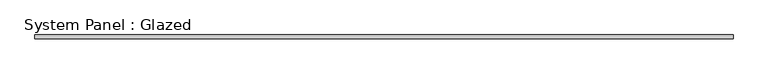
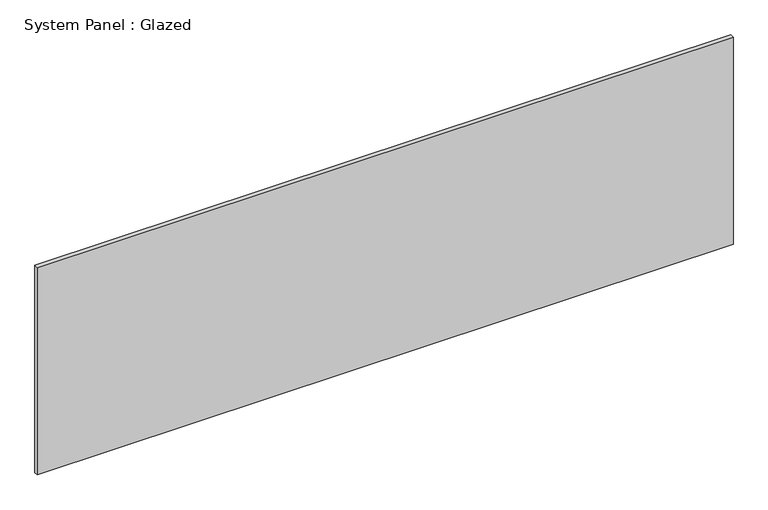
"""IFC4 building model written with IfcOpenShell, lengths in millimetres: plate geometry, System Panel : Glazed."""

from ifc_helpers import new_model, si_unit, origin, origin_with_axes, place, context, project, spatial, polyline, outline, extrude, source, transform, mapped, element, save


def system_panel_glazed_b08a8197(model_context):
    return source(origin(), model_context, "Body", "SweptSolid", [
        extrude(outline(polyline([(2321.0604018, 19.05), (-2321.0604018, 19.05), (-2321.0604018, 44.45), (2321.0604018, 44.45), (2321.0604018, 19.05)])), origin_with_axes(), (0.0, 0.0, 1.0), 1460.5),
    ])


if __name__ == "__main__":
    model = new_model("IFC4")
    model_context = context("Model", 3, world=origin())
    ifc_project = project(units=[si_unit("LENGTHUNIT", "METRE", prefix="MILLI")], contexts=[model_context])
    site = spatial("IfcSite", under=ifc_project)
    building = spatial("IfcBuilding", under=site)
    placement = place(None, origin())
    system_panel_glazed_shape = system_panel_glazed_b08a8197(model_context)
    element("IfcPlate", 1, ObjectType="System Panel : Glazed", at=placement, inside=building, context=model_context, shape_type="MappedRepresentation", body=[
        mapped(system_panel_glazed_shape, transform((0.0, 0.0, 0.0), x_axis=(1.0, 0.0, 0.0), y_axis=(0.0, 1.0, 0.0), z_axis=(0.0, 0.0, 1.0))),
    ])
    save(model, "model.ifc")

# Revit data of these elements
# Type "System Panel : Glazed"
#   Construction Type Id = "GSP4R"
#   Analytic Construction = "1/8 in Pilkington single glazing"
#   Visual Light Transmittance = 0.9
#   Solar Heat Gain Coefficient = 0.86
#   Heat Transfer Coefficient (U) = 1.18115 BTU/(h·ft²·°F)
# Element 1 (IfcPlate, "System Panel : Glazed")
#   Materials on its faces: "Glass"
# Materials
#   "Glass": class "Glass", colour RGB 0 128 192, transparency 0.75, Description = "Soda Lime Glass", Cost = 0
